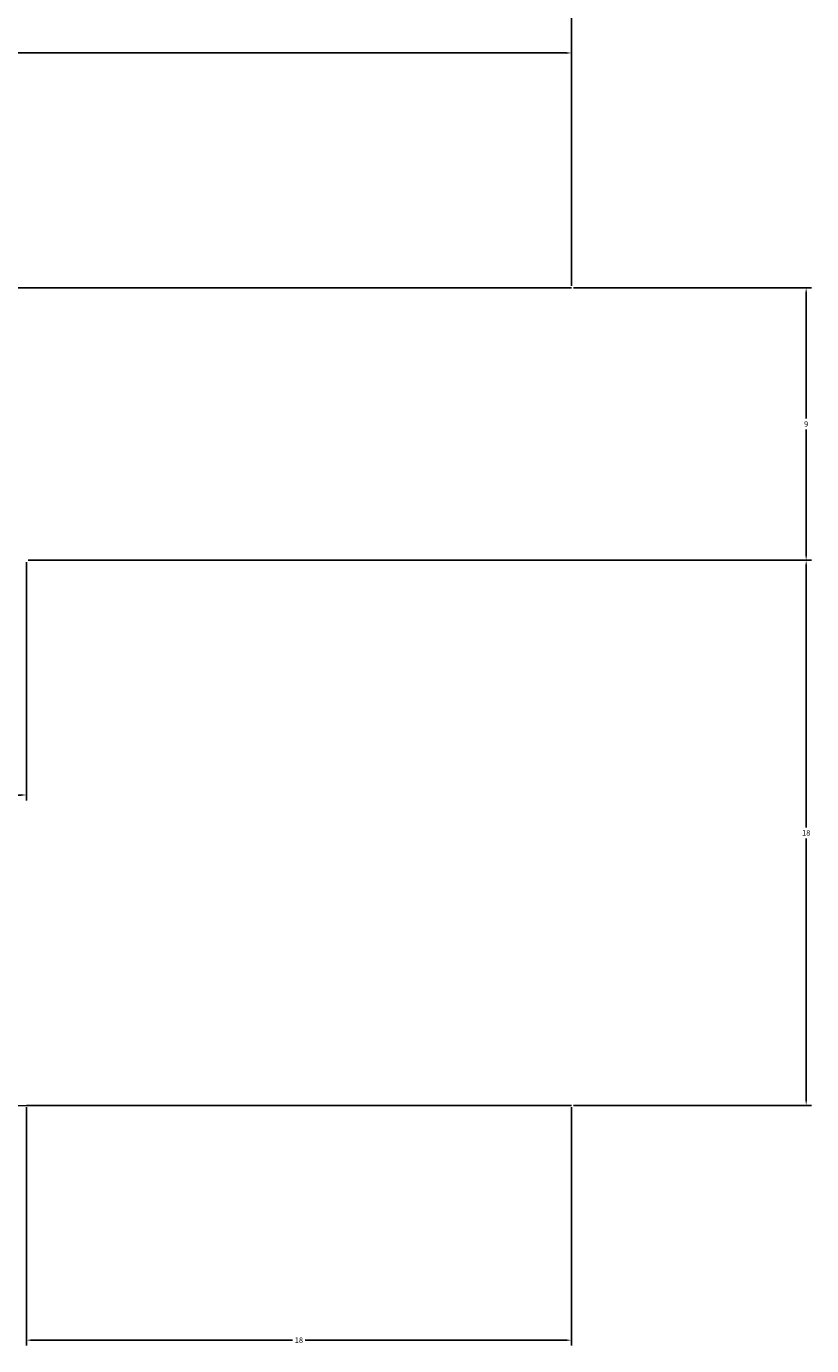
# Model space of a CAD drawing. Units: millimetres. Extents: x 223 to 381, y -8 to 62.
# Tile 4 of 5: x 355 to 381, y -8 to 36. Entities that reach past the tile are written whole.
import ezdxf

# ---------------------------------------------------------------- set-up
doc = ezdxf.new("R2010")
doc.units = ezdxf.units.MM
doc.layers.add('M-CONS', color=8, linetype='Continuous', lineweight=13)
doc.layers.add('M-DIMS', color=2, linetype='Continuous', lineweight=18)
doc.styles.get("Standard").update_dxf_attribs({"font": 'arial.ttf'})
doc.dimstyles.get("Standard").update_dxf_attribs({"dimtxt": 0.18, "dimasz": 0.18, "dimexe": 0.18, "dimexo": 0.0625, "dimgap": 0.09, "dimtad": 0, "dimtih": 1, "dimtoh": 1, "dimdec": 4, "dimzin": 0, "dimdsep": 46, "dimtxsty": 'Standard', "dimcen": 0.09, "dimadec": 0, "dimazin": 0, "dimtfac": 1, "dimtdec": 4, "dimtofl": 0, "dimtmove": 0, "dimatfit": 3, "dimfxl": 1, "dimtolj": 1, "dimtzin": 0, "dimarcsym": 0})

# ---------------------------------------------------------------- blocks, each defined once
blk = doc.blocks.new('*D1')
at = {"layer": 'Defpoints', "color": 0, "transparency": 16777216}
for p in [(372.659, 61.75), (372.659, 27), (230.659, 0)]:
    blk.add_point(p, dxfattribs=at)
at = {"layer": 'M-DIMS', "color": 0, "lineweight": -2, "transparency": 16777216}
for p, q in [((230.659, 0.062), (230.659, 61.93)), ((372.659, 27.062), (372.659, 61.93)), ((230.839, 61.75), (301.38, 61.75)), ((372.479, 61.75), (301.939, 61.75))]:
    blk.add_line(p, q, dxfattribs=at)
at = {"layer": 'M-DIMS', "color": 0, "transparency": 16777216}
for points in [[(230.839, 61.78), (230.839, 61.72), (230.659, 61.75)], [(372.479, 61.78), (372.479, 61.72), (372.659, 61.75)]]:
    blk.add_solid(points, dxfattribs=at)
at = {"layer": 'M-DIMS', "color": 0, "transparency": 16777216, "insert": (301.659, 61.75), "char_height": 0.18, "attachment_point": 5}
blk.add_mtext('\\A1;142', dxfattribs=at)
blk = doc.blocks.new('*D8')
at = {"layer": 'Defpoints', "color": 0, "transparency": 16777216}
for p in [(372.659, 34.75), (332.659, 27), (372.659, 27)]:
    blk.add_point(p, dxfattribs=at)
at = {"layer": 'M-DIMS', "color": 0, "lineweight": -2, "transparency": 16777216}
for p, q in [((332.659, 27.062), (332.659, 34.93)), ((372.659, 27.062), (372.659, 34.93)), ((332.839, 34.75), (352.437, 34.75)), ((372.479, 34.75), (352.881, 34.75))]:
    blk.add_line(p, q, dxfattribs=at)
at = {"layer": 'M-DIMS', "color": 0, "transparency": 16777216}
for points in [[(332.839, 34.78), (332.839, 34.72), (332.659, 34.75)], [(372.479, 34.78), (372.479, 34.72), (372.659, 34.75)]]:
    blk.add_solid(points, dxfattribs=at)
at = {"layer": 'M-DIMS', "color": 0, "transparency": 16777216, "insert": (352.659, 34.75), "char_height": 0.18, "attachment_point": 5}
blk.add_mtext('\\A1;40', dxfattribs=at)
blk = doc.blocks.new('*D9')
at = {"layer": 'Defpoints', "color": 0, "transparency": 16777216}
for p in [(346.324, 18), (354.659, 18), (346.324, 10.25)]:
    blk.add_point(p, dxfattribs=at)
at = {"layer": 'M-DIMS', "color": 0, "lineweight": -2, "transparency": 16777216}
for p, q in [((346.324, 17.938), (346.324, 10.07)), ((354.659, 17.938), (354.659, 10.07)), ((346.504, 10.25), (350.097, 10.25)), ((354.479, 10.25), (350.886, 10.25))]:
    blk.add_line(p, q, dxfattribs=at)
at = {"layer": 'M-DIMS', "color": 0, "transparency": 16777216}
for points in [[(346.504, 10.28), (346.504, 10.22), (346.324, 10.25)], [(354.479, 10.28), (354.479, 10.22), (354.659, 10.25)]]:
    blk.add_solid(points, dxfattribs=at)
at = {"layer": 'M-DIMS', "color": 0, "transparency": 16777216, "insert": (350.492, 10.25), "char_height": 0.18, "attachment_point": 5}
blk.add_mtext('\\A1;8.335', dxfattribs=at)
blk = doc.blocks.new('*D10')
at = {"layer": 'Defpoints', "color": 0, "transparency": 16777216}
for p in [(354.659, 0), (372.659, 0), (372.659, -7.75)]:
    blk.add_point(p, dxfattribs=at)
at = {"layer": 'M-DIMS', "color": 0, "lineweight": -2, "transparency": 16777216}
for p, q in [((354.659, -0.062), (354.659, -7.93)), ((372.659, -0.062), (372.659, -7.93)), ((354.839, -7.75), (363.449, -7.75)), ((372.479, -7.75), (363.87, -7.75))]:
    blk.add_line(p, q, dxfattribs=at)
at = {"layer": 'M-DIMS', "color": 0, "transparency": 16777216}
for points in [[(354.839, -7.72), (354.839, -7.78), (354.659, -7.75)], [(372.479, -7.72), (372.479, -7.78), (372.659, -7.75)]]:
    blk.add_solid(points, dxfattribs=at)
at = {"layer": 'M-DIMS', "color": 0, "transparency": 16777216, "insert": (363.659, -7.75), "char_height": 0.18, "attachment_point": 5}
blk.add_mtext('\\A1;18', dxfattribs=at)
blk = doc.blocks.new('*D12')
at = {"layer": 'Defpoints', "color": 0, "transparency": 16777216}
for p in [(354.659, 18), (380.409, 18), (372.659, 0)]:
    blk.add_point(p, dxfattribs=at)
at = {"layer": 'M-DIMS', "color": 0, "lineweight": -2, "transparency": 16777216}
for p, q in [((354.722, 18), (380.589, 18)), ((380.409, 17.82), (380.409, 9.182)), ((380.409, 0.18), (380.409, 8.818)), ((372.722, 0), (380.589, 0))]:
    blk.add_line(p, q, dxfattribs=at)
at = {"layer": 'M-DIMS', "color": 0, "transparency": 16777216}
for points in [[(380.379, 17.82), (380.439, 17.82), (380.409, 18)], [(380.379, 0.18), (380.439, 0.18), (380.409, 0)]]:
    blk.add_solid(points, dxfattribs=at)
at = {"layer": 'M-DIMS', "color": 0, "transparency": 16777216, "insert": (380.409, 9), "char_height": 0.18, "attachment_point": 5}
blk.add_mtext('\\A1;18', dxfattribs=at)
blk = doc.blocks.new('*D13')
at = {"layer": 'Defpoints', "color": 0, "transparency": 16777216}
for p in [(372.659, 27), (380.409, 27), (354.659, 18)]:
    blk.add_point(p, dxfattribs=at)
at = {"layer": 'M-DIMS', "color": 0, "lineweight": -2, "transparency": 16777216}
for p, q in [((372.722, 27), (380.589, 27)), ((380.409, 26.82), (380.409, 22.682)), ((380.409, 18.18), (380.409, 22.318)), ((354.722, 18), (380.589, 18))]:
    blk.add_line(p, q, dxfattribs=at)
at = {"layer": 'M-DIMS', "color": 0, "transparency": 16777216}
for points in [[(380.379, 26.82), (380.439, 26.82), (380.409, 27)], [(380.379, 18.18), (380.439, 18.18), (380.409, 18)]]:
    blk.add_solid(points, dxfattribs=at)
at = {"layer": 'M-DIMS', "color": 0, "transparency": 16777216, "insert": (380.409, 22.5), "char_height": 0.18, "attachment_point": 5}
blk.add_mtext('\\A1;9', dxfattribs=at)

msp = doc.modelspace()

# ---------------------------------------------------------------- linework, layer by layer
at = {"layer": 'M-CONS', "extrusion": (0, -1, 0)}
for p, q in [((332.6592, 0, 103.6363), (372.6592, 0, 103.6363)), ((372.6592, 0, 63.6363), (354.6592, 0, 63.6363)), ((372.6592, 0, 103.6363), (372.6592, 0, 63.6363))]:
    msp.add_line(p, q, dxfattribs=at)
at = {"layer": 'M-CONS'}
msp.add_polyline3d([(332.6592, 27, 103.6363), (372.6592, 27, 143.6363), (372.6592, 27, 103.6363)], close=True, dxfattribs=at)

# ---------------------------------------------------------------- dimensions: what is measured, and where the dimension line sits
at = {"layer": 'M-DIMS'}
for base, p1, p2, picture, middle in [((372.6592, 61.75), (230.6592, 0), (372.6592, 27), '*D1', (301.6592, 61.75)), ((372.6592, 34.75), (332.6592, 27), (372.6592, 27), '*D8', (352.6592, 34.75)), ((372.6592, -7.75), (354.6592, 0), (372.6592, 0), '*D10', (363.6592, -7.75))]:
    dim = msp.add_linear_dim(base=base, p1=p1, p2=p2, dimstyle='Standard', override={"dimdec": 0, "dimlfac": 1, "dimrnd": 0, "dimzin": 0, "dimdsep": 46, "dimlunit": 2}, dxfattribs=at)
    dim.commit()
    dim.dimension.update_dxf_attribs({"geometry": picture, "text_midpoint": middle})
for base, p1, p2, angle, override, picture, middle in [((380.4092, 27), (354.6592, 18), (372.6592, 27), 90, {"dimdec": 0, "dimlfac": 1, "dimrnd": 0, "dimzin": 0, "dimdsep": 46, "dimlunit": 2}, '*D13', (380.4092, 22.5)), ((346.324, 10.25), (354.6592, 18), (346.324, 18), 180, {"dimdec": 3, "dimlfac": 1, "dimrnd": 0, "dimzin": 0, "dimdsep": 46, "dimlunit": 2}, '*D9', (350.4916, 10.25)), ((380.4092, 18), (372.6592, 0), (354.6592, 18), 90, {"dimdec": 0, "dimlfac": 1, "dimrnd": 0, "dimzin": 0, "dimdsep": 46, "dimlunit": 2}, '*D12', (380.4092, 9))]:
    dim = msp.add_linear_dim(base=base, p1=p1, p2=p2, angle=angle, dimstyle='Standard', override=override, dxfattribs=at)
    dim.commit()
    dim.dimension.update_dxf_attribs({"geometry": picture, "text_midpoint": middle})

doc.saveas('drawing.dxf')
